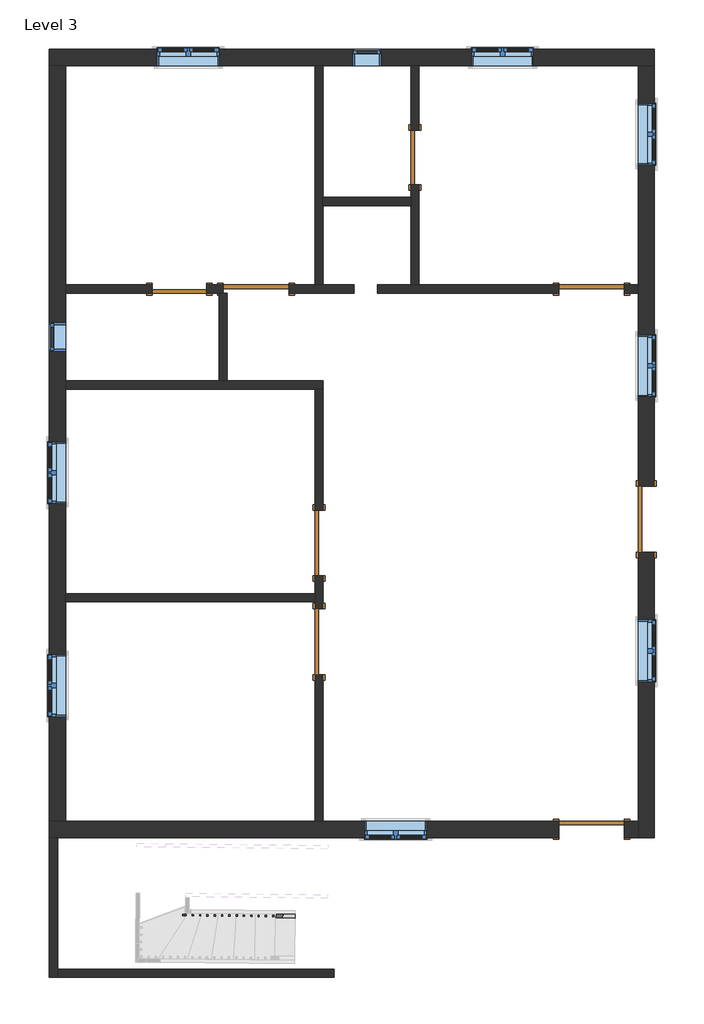
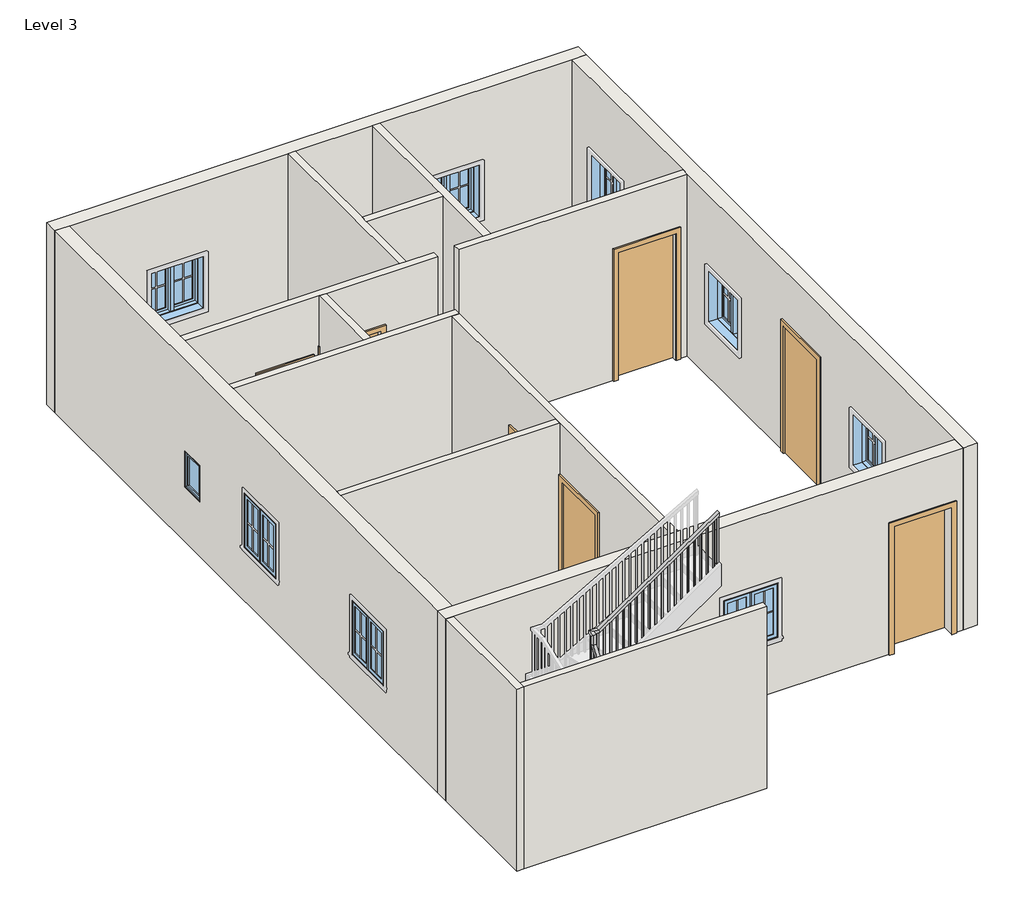
# One storey, part 1 of 2: 15 walls, 10 windows, 8 doors, 1 railing.
"""IFC4 building model written with IfcOpenShell, lengths in millimetres."""

from ifc_helpers import new_model, si_unit, frame, origin, place, context, project, spatial, polyline, outline, extrude, faceted_brep, transform, mapped, element, save
from components import door_f2b275c1, door_e5f9f3c4, door_305aa2a5, door_a90ba1ad, door_0ca8825f, window_aa618e30, window_339605e1

model = new_model("IFC4")

# Units and contexts
model_context = context("Model", 3, world=origin())
ifc_project = project(units=[si_unit("LENGTHUNIT", "METRE", prefix="MILLI")], contexts=[model_context])

# Site, building, storey
site = spatial("IfcSite", under=ifc_project)
building = spatial("IfcBuilding", under=site)
storey = spatial("IfcBuildingStorey", under=building, Name="Level 3", Elevation=3200.4)

# Doors
placement = place(None, origin())
door_shape = door_f2b275c1(model_context)
element("IfcDoor", 1, ObjectType="Single-Flush : 30\" x 80\"", at=placement, inside=storey, context=model_context, shape_type="MappedRepresentation", body=[
    mapped(door_shape, transform((-295.4747832, 5557.2532079, 3200.4), x_axis=(0.0, -1.0, 0.0), y_axis=(1.0, 0.0, 0.0), z_axis=(0.0, 0.0, 1.0))),
])
element("IfcDoor", 2, ObjectType="Single-Flush : 30\" x 80\"", at=placement, inside=storey, context=model_context, shape_type="MappedRepresentation", body=[
    mapped(door_shape, transform((-3572.0747832, 3728.4532079, 3200.4), x_axis=(1.0, 0.0, 0.0), y_axis=(0.0, 1.0, 0.0), z_axis=(0.0, 0.0, 1.0))),
])
door_2_shape = door_e5f9f3c4(model_context)
element("IfcDoor", 3, ObjectType="Single-Flush : 36\" x 84\"", at=placement, inside=storey, context=model_context, shape_type="MappedRepresentation", body=[
    mapped(door_2_shape, transform((-2505.2747832, 3728.4532079, 3200.4), x_axis=(1.0, 0.0, 0.0), y_axis=(0.0, 1.0, 0.0), z_axis=(0.0, 0.0, 1.0))),
])
element("IfcDoor", 4, ObjectType="Single-Flush : 36\" x 84\"", at=placement, inside=storey, context=model_context, shape_type="MappedRepresentation", body=[
    mapped(door_2_shape, transform((2161.9752168, 3728.4532079, 3200.4), x_axis=(1.0, 0.0, 0.0), y_axis=(0.0, 1.0, 0.0), z_axis=(0.0, 0.0, 1.0))),
])
element("IfcDoor", 5, ObjectType="Single-Flush : 36\" x 84\"", at=placement, inside=storey, context=model_context, shape_type="MappedRepresentation", body=[
    mapped(door_2_shape, transform((-1628.9747832, -1173.7467921, 3200.4), x_axis=(0.0, 1.0, 0.0), y_axis=(-1.0, 0.0, 0.0), z_axis=(0.0, 0.0, 1.0))),
])
door_3_shape = door_305aa2a5(model_context)
element("IfcDoor", 6, ObjectType="Single-Flush : 36\" x 84\"", at=placement, inside=storey, context=model_context, shape_type="MappedRepresentation", body=[
    mapped(door_3_shape, transform((-1628.9747832, 197.8532079, 3200.4), x_axis=(0.0, -1.0, 0.0), y_axis=(1.0, 0.0, 0.0), z_axis=(0.0, 0.0, 1.0))),
])
door_4_shape = door_a90ba1ad(model_context)
element("IfcDoor", 7, ObjectType="Single-Flush : 36\" x 84\"", at=placement, inside=storey, context=model_context, shape_type="MappedRepresentation", body=[
    mapped(door_4_shape, transform((2923.9752168, 528.0532079, 3200.4), x_axis=(0.0, -1.0, 0.0), y_axis=(1.0, 0.0, 0.0), z_axis=(0.0, 0.0, 1.0))),
])
door_5_shape = door_0ca8825f(model_context)
element("IfcDoor", 8, ObjectType="Single-Flush : 36\" x 84\"", at=placement, inside=storey, context=model_context, shape_type="MappedRepresentation", body=[
    mapped(door_5_shape, transform((2161.9752168, -3783.5967921, 3200.4), x_axis=(1.0, 0.0, 0.0), y_axis=(0.0, 1.0, 0.0), z_axis=(0.0, 0.0, 1.0))),
])

# Railing
element("IfcRailing", 9, ObjectType="Handrail - Rectangular", at=placement, inside=storey, context=model_context, shape_type="SolidModel", body=[
    faceted_brep([(-1962.1803506, -5016.2038017, 4284.1333333), (-1962.1803506, -5016.2038017, 4222.6793596), (-1961.6349602, -4965.4067295, 4222.6793596), (-1961.6349602, -4965.4067295, 4284.1333333), (-3413.6283866, -5000.6201116, 5272.2756169), (-3464.4254588, -5000.0747212, 5245.4041661), (-3463.8800684, -4949.2776489, 5245.4041661), (-3413.0829962, -4949.8230393, 5272.2756169), (-3413.6283866, -5000.6201116, 5489.361538), (-3464.4254588, -5000.0747212, 5438.561538), (-3463.8800684, -4949.2776489, 5438.561538), (-3413.0829962, -4949.8230393, 5489.361538), (-3540.6210672, -4999.2566356, 5489.361538), (-3540.6210672, -4999.2566356, 5438.561538), (-3489.2786045, -4949.0049537, 5438.561538), (-3489.2786045, -4949.0049537, 5489.361538), (-3539.2575912, -4872.2639549, 5489.361538), (-3538.9677931, -4845.272478, 5438.561538), (-3488.1707209, -4845.8178684, 5438.561538), (-3488.4605189, -4872.8093453, 5489.361538), (-3537.8941152, -4745.2712743, 5677.4249579), (-3537.3487248, -4694.4742021, 5661.8786564), (-3486.5516525, -4695.0195925, 5661.8786564), (-3487.0970429, -4745.8166647, 5677.4249579), (-3537.8941152, -4745.2712743, 5845.476961), (-3537.3487248, -4694.4742021, 5794.676961), (-3486.5516525, -4695.0195925, 5794.676961), (-3487.0970429, -4745.8166647, 5845.476961), (-3536.5306392, -4618.2785937, 5845.476961), (-3536.5306392, -4618.2785937, 5794.676961), (-3486.2789573, -4669.6210563, 5794.676961), (-3486.2789573, -4669.6210563, 5845.476961), (-3409.5379585, -4619.6420697, 5845.476961), (-3393.6525863, -4619.8126254, 5794.676961), (-3394.1979767, -4670.6096976, 5794.676961), (-3410.0833489, -4670.439142, 5845.476961), (-1509.4062983, -4640.0431191, 7162.8), (-1509.9516887, -4690.8401913, 7162.8), (-1509.9516887, -4690.8401913, 7100.9869912), (-1509.4062983, -4640.0431191, 7100.9869912)], [[[0, 1, 2, 3]], [[1, 0, 4, 5]], [[2, 1, 5, 6]], [[3, 2, 6, 7]], [[0, 3, 7, 4]], [[5, 4, 8, 9]], [[6, 5, 9, 10]], [[7, 6, 10, 11]], [[4, 7, 11, 8]], [[9, 8, 12, 13]], [[10, 9, 13, 14]], [[11, 10, 14, 15]], [[8, 11, 15, 12]], [[13, 12, 16, 17]], [[14, 13, 17, 18]], [[15, 14, 18, 19]], [[12, 15, 19, 16]], [[17, 16, 20, 21]], [[18, 17, 21, 22]], [[19, 18, 22, 23]], [[16, 19, 23, 20]], [[21, 20, 24, 25]], [[22, 21, 25, 26]], [[23, 22, 26, 27]], [[20, 23, 27, 24]], [[25, 24, 28, 29]], [[26, 25, 29, 30]], [[27, 26, 30, 31]], [[24, 27, 31, 28]], [[29, 28, 32, 33]], [[30, 29, 33, 34]], [[31, 30, 34, 35]], [[28, 31, 35, 32]], [[36, 37, 38, 39]], [[33, 32, 36, 39]], [[34, 33, 39, 38]], [[35, 34, 38, 37]], [[32, 35, 37, 36]]]),
    extrude(outline(polyline([(221.9968897, -19.05), (235.2031102, 0.0), (1200.994449, 0.0), (1200.994449, -19.05), (221.9968897, -19.05)])), frame((-1590.7427644, -4674.0968508, 7280.0611157), z_axis=(0.01073603161956521, 0.9999423671517594, 0.0), x_axis=(0.0, 0.0, -1.0)), (0.0, 0.0, 1.0), 19.05),
    extrude(outline(polyline([(221.9968898, -19.05), (235.2031102, 0.0), (1130.5612733, 0.0), (1130.5612733, -19.05), (221.9968898, -19.05)])), frame((-1692.3369089, -4673.00607, 7209.62794), z_axis=(0.01073603161956521, 0.9999423671517594, 0.0), x_axis=(0.0, 0.0, -1.0)), (0.0, 0.0, 1.0), 19.05),
    extrude(outline(polyline([(221.9968897, -19.05), (235.2031102, 0.0), (1060.1280975, 0.0), (1060.1280975, -19.05), (221.9968897, -19.05)])), frame((-1793.9310534, -4671.9152892, 7139.1947642), z_axis=(0.01073603161956521, 0.9999423671517594, 0.0), x_axis=(0.0, 0.0, -1.0)), (0.0, 0.0, 1.0), 19.05),
    extrude(outline(polyline([(221.9968898, -19.05), (235.2031103, 0.0), (1159.0282552, 0.0), (1159.0282552, -19.05), (221.9968898, -19.05)])), frame((-1895.5251979, -4670.8245084, 7068.7615885), z_axis=(0.01073603161956521, 0.9999423671517594, 0.0), x_axis=(0.0, 0.0, -1.0)), (0.0, 0.0, 1.0), 19.05),
    extrude(outline(polyline([(221.9968898, -19.05), (235.2031102, 0.0), (1088.5950794, 0.0), (1088.5950794, -19.05), (221.9968898, -19.05)])), frame((-1997.1193424, -4669.7337275, 6998.3284127), z_axis=(0.01073603161956521, 0.9999423671517594, 0.0), x_axis=(0.0, 0.0, -1.0)), (0.0, 0.0, 1.0), 19.05),
    extrude(outline(polyline([(221.9968898, -19.05), (235.2031103, 0.0), (1187.495237, 0.0), (1187.495237, -19.05), (221.9968898, -19.05)])), frame((-2098.7134869, -4668.6429467, 6927.895237), z_axis=(0.01073603161956521, 0.9999423671517594, 0.0), x_axis=(0.0, 0.0, -1.0)), (0.0, 0.0, 1.0), 19.05),
    extrude(outline(polyline([(221.9968898, -19.05), (235.2031102, 0.0), (1117.0620612, 0.0), (1117.0620612, -19.05), (221.9968898, -19.05)])), frame((-2200.3076314, -4667.5521659, 6857.4620612), z_axis=(0.01073603161956521, 0.9999423671517594, 0.0), x_axis=(0.0, 0.0, -1.0)), (0.0, 0.0, 1.0), 19.05),
    extrude(outline(polyline([(221.9968897, -19.0499999), (235.2031102, 0.0), (1046.6288854, 0.0), (1046.6288854, -19.0499999), (221.9968897, -19.0499999)])), frame((-2301.9017759, -4666.4613851, 6787.0288854), z_axis=(0.01073603161956521, 0.9999423671517594, 0.0), x_axis=(0.0, 0.0, -1.0)), (0.0, 0.0, 1.0), 19.05),
    extrude(outline(polyline([(221.9968898, -19.0499999), (235.2031102, 0.0), (1145.529043, 0.0), (1145.529043, -19.0499999), (221.9968898, -19.0499999)])), frame((-2403.4959204, -4665.3706043, 6716.5957097), z_axis=(0.01073603161956521, 0.9999423671517594, 0.0), x_axis=(0.0, 0.0, -1.0)), (0.0, 0.0, 1.0), 19.05),
    extrude(outline(polyline([(221.9968897, -19.05), (235.2031102, 0.0), (1075.0958672, 0.0), (1075.0958672, -19.05), (221.9968897, -19.05)])), frame((-2505.090065, -4664.2798235, 6646.1625339), z_axis=(0.01073603161956521, 0.9999423671517594, 0.0), x_axis=(0.0, 0.0, -1.0)), (0.0, 0.0, 1.0), 19.05),
    extrude(outline(polyline([(221.9968898, -19.05), (235.2031103, 0.0), (1004.6626915, 0.0), (1004.6626915, -19.05), (221.9968898, -19.05)])), frame((-2606.6842095, -4663.1890427, 6575.7293582), z_axis=(0.01073603161956521, 0.9999423671517594, 0.0), x_axis=(0.0, 0.0, -1.0)), (0.0, 0.0, 1.0), 19.05),
    extrude(outline(polyline([(221.9968898, -19.05), (235.2031102, 0.0), (1103.5628491, 0.0), (1103.5628491, -19.05), (221.9968898, -19.05)])), frame((-2708.278354, -4662.0982619, 6505.2961824), z_axis=(0.01073603161956521, 0.9999423671517594, 0.0), x_axis=(0.0, 0.0, -1.0)), (0.0, 0.0, 1.0), 19.05),
    extrude(outline(polyline([(221.9968898, -19.05), (235.2031103, 0.0), (1033.1296734, 0.0), (1033.1296734, -19.05), (221.9968898, -19.05)])), frame((-2809.8724985, -4661.007481, 6434.8630067), z_axis=(0.01073603161956521, 0.9999423671517594, 0.0), x_axis=(0.0, 0.0, -1.0)), (0.0, 0.0, 1.0), 19.05),
    extrude(outline(polyline([(221.9968898, -19.05), (235.2031102, 0.0), (1132.0298309, 0.0), (1132.0298309, -19.05), (221.9968898, -19.05)])), frame((-2911.466643, -4659.9167002, 6364.4298309), z_axis=(0.01073603161956521, 0.9999423671517594, 0.0), x_axis=(0.0, 0.0, -1.0)), (0.0, 0.0, 1.0), 19.05),
    extrude(outline(polyline([(221.9968897, -19.05), (235.2031102, 0.0), (1061.5966551, 0.0), (1061.5966551, -19.05), (221.9968897, -19.05)])), frame((-3013.0607875, -4658.8259194, 6293.9966551), z_axis=(0.01073603161956521, 0.9999423671517594, 0.0), x_axis=(0.0, 0.0, -1.0)), (0.0, 0.0, 1.0), 19.05),
    extrude(outline(polyline([(221.9968898, -19.05), (235.2031102, 0.0), (991.1634794, 0.0), (991.1634794, -19.05), (221.9968898, -19.05)])), frame((-3114.654932, -4657.7351386, 6223.5634794), z_axis=(0.01073603161956521, 0.9999423671517594, 0.0), x_axis=(0.0, 0.0, -1.0)), (0.0, 0.0, 1.0), 19.05),
    extrude(outline(polyline([(221.9968897, -19.05), (235.2031102, 0.0), (1090.0636369, 0.0), (1090.0636369, -19.05), (221.9968897, -19.05)])), frame((-3216.2490765, -4656.6443578, 6153.1303036), z_axis=(0.01073603161956521, 0.9999423671517594, 0.0), x_axis=(0.0, 0.0, -1.0)), (0.0, 0.0, 1.0), 19.05),
    extrude(outline(polyline([(221.9968898, -19.05), (235.2031103, 0.0), (1019.6304612, 0.0), (1019.6304612, -19.05), (221.9968898, -19.05)])), frame((-3317.843221, -4655.553577, 6082.6971279), z_axis=(0.01073603161956521, 0.9999423671517594, 0.0), x_axis=(0.0, 0.0, -1.0)), (0.0, 0.0, 1.0), 19.05),
    extrude(outline(polyline([(221.9968898, -19.05), (235.2031102, 0.0), (1118.5306188, 0.0), (1118.5306188, -19.05), (221.9968898, -19.05)])), frame((-3419.4373655, -4654.4627962, 6012.2639521), z_axis=(0.01073603161956521, 0.9999423671517594, 0.0), x_axis=(0.0, 0.0, -1.0)), (0.0, 0.0, 1.0), 19.05),
    extrude(outline(polyline([(-3502.2553031, -4678.9750729), (-3521.3042052, -4678.7705515), (-3521.0996838, -4659.7216494), (-3502.0507817, -4659.9261708), (-3502.2553031, -4678.9750729)])), frame((0.0, 0.0, 4724.4), z_axis=(0.0, 0.0, 1.0), x_axis=(1.0, 0.0, 0.0)), (0.0, 0.0, 1.0), 1070.276961),
    extrude(outline(polyline([(214.4952435, -19.05), (242.7047565, 0.0), (1222.5739377, 0.0), (1222.5739377, -19.05), (214.4952435, -19.05)])), frame((-3503.3460839, -4780.5692174, 5777.6406044), z_axis=(-0.9999423671517594, 0.010736031619565895, 0.0), x_axis=(0.0, 0.0, -1.0)), (0.0, 0.0, 1.0), 19.05),
    extrude(outline(polyline([(214.4952435, -19.05), (242.7047565, 0.0), (1072.1232018, 0.0), (1072.1232018, -19.05), (214.4952435, -19.05)])), frame((-3504.4368647, -4882.1633619, 5627.1898685), z_axis=(-0.9999423671517594, 0.010736031619565895, 0.0), x_axis=(0.0, 0.0, -1.0)), (0.0, 0.0, 1.0), 19.05),
    extrude(outline(polyline([(-3476.1931112, -4965.0213631), (-3476.3976326, -4984.0702652), (-3495.4465347, -4983.8657438), (-3495.2420133, -4964.8168417), (-3476.1931112, -4965.0213631)])), frame((0.0, 0.0, 4385.7333333), z_axis=(0.0, 0.0, 1.0), x_axis=(1.0, 0.0, 0.0)), (0.0, 0.0, 1.0), 1052.8282047),
    extrude(outline(polyline([(235.0842231, -19.05), (222.115777, 0.0), (1203.1900014, 0.0), (1203.1900014, -19.05), (235.0842231, -19.05)])), frame((-3393.8523902, -4984.9565246, 5419.5900014), z_axis=(0.01073603161956537, 0.9999423671517593, 0.0), x_axis=(0.0, 0.0, -1.0)), (0.0, 0.0, 1.0), 19.05),
    extrude(outline(polyline([(235.084223, -19.05), (222.1157769, 0.0), (1134.0249555, 0.0), (1134.0249555, -19.05), (235.084223, -19.05)])), frame((-3292.2582457, -4986.0473054, 5350.4249555), z_axis=(0.01073603161956537, 0.9999423671517593, 0.0), x_axis=(0.0, 0.0, -1.0)), (0.0, 0.0, 1.0), 19.05),
    extrude(outline(polyline([(235.0842231, -19.05), (222.115777, 0.0), (1234.193243, 0.0), (1234.193243, -19.05), (235.0842231, -19.05)])), frame((-3190.6641012, -4987.1380862, 5281.2599097), z_axis=(0.01073603161956537, 0.9999423671517593, 0.0), x_axis=(0.0, 0.0, -1.0)), (0.0, 0.0, 1.0), 19.05),
    extrude(outline(polyline([(235.084223, -19.05), (222.1157769, 0.0), (1165.0281971, 0.0), (1165.0281971, -19.05), (235.084223, -19.05)])), frame((-3089.0699567, -4988.228867, 5212.0948638), z_axis=(0.01073603161956537, 0.9999423671517593, 0.0), x_axis=(0.0, 0.0, -1.0)), (0.0, 0.0, 1.0), 19.05),
    extrude(outline(polyline([(235.084223, -19.05), (222.1157769, 0.0), (1265.1964847, 0.0), (1265.1964847, -19.05), (235.084223, -19.05)])), frame((-2987.4758122, -4989.3196478, 5142.929818), z_axis=(0.01073603161956537, 0.9999423671517593, 0.0), x_axis=(0.0, 0.0, -1.0)), (0.0, 0.0, 1.0), 19.05),
    extrude(outline(polyline([(235.0842231, -19.05), (222.115777, 0.0), (1196.0314389, 0.0), (1196.0314389, -19.05), (235.0842231, -19.05)])), frame((-2885.8816677, -4990.4104286, 5073.7647722), z_axis=(0.01073603161956537, 0.9999423671517593, 0.0), x_axis=(0.0, 0.0, -1.0)), (0.0, 0.0, 1.0), 19.05),
    extrude(outline(polyline([(235.084223, -19.05), (222.1157769, 0.0), (1296.1997263, 0.0), (1296.1997263, -19.05), (235.084223, -19.05)])), frame((-2784.2875232, -4991.5012094, 5004.5997263), z_axis=(0.01073603161956537, 0.9999423671517593, 0.0), x_axis=(0.0, 0.0, -1.0)), (0.0, 0.0, 1.0), 19.05),
    extrude(outline(polyline([(235.0842231, -19.05), (222.115777, 0.0), (1227.0346805, 0.0), (1227.0346805, -19.05), (235.0842231, -19.05)])), frame((-2682.6933787, -4992.5919903, 4935.4346805), z_axis=(0.01073603161956537, 0.9999423671517593, 0.0), x_axis=(0.0, 0.0, -1.0)), (0.0, 0.0, 1.0), 19.05),
    extrude(outline(polyline([(235.084223, -19.05), (222.1157769, 0.0), (1157.8696346, 0.0), (1157.8696346, -19.05), (235.084223, -19.05)])), frame((-2581.0992342, -4993.6827711, 4866.2696346), z_axis=(0.01073603161956537, 0.9999423671517593, 0.0), x_axis=(0.0, 0.0, -1.0)), (0.0, 0.0, 1.0), 19.05),
    extrude(outline(polyline([(235.0842231, -19.05), (222.115777, 0.0), (1258.0379221, 0.0), (1258.0379221, -19.05), (235.0842231, -19.05)])), frame((-2479.5050897, -4994.7735519, 4797.1045888), z_axis=(0.01073603161956537, 0.9999423671517593, 0.0), x_axis=(0.0, 0.0, -1.0)), (0.0, 0.0, 1.0), 19.05),
    extrude(outline(polyline([(235.084223, -19.05), (222.1157769, 0.0), (1188.8728762, 0.0), (1188.8728762, -19.05), (235.084223, -19.05)])), frame((-2377.9109452, -4995.8643327, 4727.9395429), z_axis=(0.01073603161956537, 0.9999423671517593, 0.0), x_axis=(0.0, 0.0, -1.0)), (0.0, 0.0, 1.0), 19.05),
    extrude(outline(polyline([(235.084223, -19.05), (222.115777, 0.0), (1119.7078304, 0.0), (1119.7078304, -19.05), (235.084223, -19.05)])), frame((-2276.3168007, -4996.9551135, 4658.7744971), z_axis=(0.01073603161956537, 0.9999423671517593, 0.0), x_axis=(0.0, 0.0, -1.0)), (0.0, 0.0, 1.0), 19.05),
    extrude(outline(polyline([(235.0842231, -19.05), (222.115777, 0.0), (1219.876118, 0.0), (1219.876118, -19.05), (235.0842231, -19.05)])), frame((-2174.7226562, -4998.0458943, 4589.6094513), z_axis=(0.01073603161956537, 0.9999423671517593, 0.0), x_axis=(0.0, 0.0, -1.0)), (0.0, 0.0, 1.0), 19.05),
    extrude(outline(polyline([(235.084223, -19.05), (222.1157769, 0.0), (1150.7110721, 0.0), (1150.7110721, -19.05), (235.084223, -19.05)])), frame((-2073.1285117, -4999.1366751, 4520.4444054), z_axis=(0.01073603161956537, 0.9999423671517593, 0.0), x_axis=(0.0, 0.0, -1.0)), (0.0, 0.0, 1.0), 19.05),
    extrude(outline(polyline([(-3501.9826079, -4653.5765368), (-3521.03151, -4653.3720154), (-3520.8269886, -4634.3231133), (-3501.7780865, -4634.5276347), (-3501.9826079, -4653.5765368)])), frame((0.0, 0.0, 4724.4), z_axis=(0.0, 0.0, 1.0), x_axis=(1.0, 0.0, 0.0)), (0.0, 0.0, 1.0), 1070.276961),
    extrude(outline(polyline([(-3505.3231241, -4964.7086043), (-3505.5276455, -4983.7575064), (-3524.5765476, -4983.552985), (-3524.3720262, -4964.5040829), (-3505.3231241, -4964.7086043)])), frame((0.0, 0.0, 4385.7333333), z_axis=(0.0, 0.0, 1.0), x_axis=(1.0, 0.0, 0.0)), (0.0, 0.0, 1.0), 1052.8282047),
    extrude(outline(polyline([(221.9968897, -19.05), (235.2031102, 0.0), (1243.9172142, 0.0), (1243.9172142, -19.05), (221.9968897, -19.05)])), frame((-1528.8301563, -4674.7615848, 7322.9838809), z_axis=(0.01073603161956521, 0.9999423671517594, 0.0), x_axis=(0.0, 0.0, -1.0)), (0.0, 0.0, 1.0), 19.05),
    extrude(outline(polyline([(235.084223, -19.05), (222.1157769, 0.0), (1088.0302493, 0.0), (1088.0302493, -19.05), (235.084223, -19.05)])), frame((-1981.0588182, -5000.1251952, 4457.7635826), z_axis=(0.01073603161956537, 0.9999423671517593, 0.0), x_axis=(0.0, 0.0, -1.0)), (0.0, 0.0, 1.0), 19.05),
])

# Walls
element("IfcWall", 10, ObjectType="WALL4.5\"", at=placement, inside=storey, context=model_context, shape_type="Brep", body=[
    faceted_brep([(-2048.0747832, 3671.3032079, 5334.0), (-2048.0747832, 3671.3032079, 3200.4), (-1141.0287494, 3671.3032079, 3200.4), (-1141.0287494, 3671.3032079, 6248.4), (-2905.3247832, 3671.3032079, 6248.4), (-3019.6247832, 3671.3032079, 6248.4), (-5153.2247832, 3671.3032079, 6248.4), (-5153.2247832, 3671.3032079, 3200.4), (-3953.0747832, 3671.3032079, 3200.4), (-3953.0747832, 3671.3032079, 5232.4), (-3191.0747832, 3671.3032079, 5232.4), (-3191.0747832, 3671.3032079, 3200.4), (-3019.6247832, 3671.3032079, 3200.4), (-2962.4747832, 3671.3032079, 3200.4), (-2962.4747832, 3671.3032079, 5334.0), (-1141.0287494, 3785.6032079, 3200.4), (-1571.8247832, 3785.6032079, 3200.4), (-1686.1247832, 3785.6032079, 3200.4), (-2048.0747832, 3785.6032079, 3200.4), (-2048.0747832, 3785.6032079, 5334.0), (-2962.4747832, 3785.6032079, 5334.0), (-2962.4747832, 3785.6032079, 3200.4), (-3191.0747832, 3785.6032079, 3200.4), (-3191.0747832, 3785.6032079, 5232.4), (-3953.0747832, 3785.6032079, 5232.4), (-3953.0747832, 3785.6032079, 3200.4), (-5153.2247832, 3785.6032079, 3200.4), (-5153.2247832, 3785.6032079, 6248.4), (-1686.1247832, 3785.6032079, 6248.4), (-1571.8247832, 3785.6032079, 6248.4), (-1141.0287494, 3785.6032079, 6248.4)], [[[0, 1, 2, 3, 4, 5, 6, 7, 8, 9, 10, 11, 12, 13, 14]], [[15, 16, 17, 18, 19, 20, 21, 22, 23, 24, 25, 26, 27, 28, 29, 30]], [[8, 7, 26, 25]], [[2, 1, 18, 17, 16, 15]], [[13, 12, 11, 22, 21]], [[3, 2, 15, 30]], [[7, 6, 27, 26]], [[23, 22, 11, 10]], [[24, 23, 10, 9]], [[25, 24, 9, 8]], [[19, 18, 1, 0]], [[20, 19, 0, 14]], [[21, 20, 14, 13]], [[6, 5, 4, 3, 30, 29, 28, 27]]]),
])
element("IfcWall", 11, ObjectType="WALL4.5\"", at=placement, inside=storey, context=model_context, shape_type="Brep", body=[
    faceted_brep([(2619.1752168, 3671.3032079, 5334.0), (2619.1752168, 3671.3032079, 3200.4), (2809.6752168, 3671.3032079, 3200.4), (2809.6752168, 3671.3032079, 6248.4), (-812.7163761, 3671.3032079, 6248.4), (-812.7163761, 3671.3032079, 3200.4), (1704.7752168, 3671.3032079, 3200.4), (1704.7752168, 3671.3032079, 5334.0), (2809.6752168, 3785.6032079, 3200.4), (2619.1752168, 3785.6032079, 3200.4), (2619.1752168, 3785.6032079, 5334.0), (1704.7752168, 3785.6032079, 5334.0), (1704.7752168, 3785.6032079, 3200.4), (-238.3247832, 3785.6032079, 3200.4), (-352.6247832, 3785.6032079, 3200.4), (-812.7163761, 3785.6032079, 3200.4), (-812.7163761, 3785.6032079, 6248.4), (-352.6247832, 3785.6032079, 6248.4), (-238.3247832, 3785.6032079, 6248.4), (2809.6752168, 3785.6032079, 6248.4)], [[[0, 1, 2, 3, 4, 5, 6, 7]], [[8, 9, 10, 11, 12, 13, 14, 15, 16, 17, 18, 19]], [[6, 5, 15, 14, 13, 12]], [[2, 1, 9, 8]], [[5, 4, 16, 15]], [[3, 2, 8, 19]], [[10, 9, 1, 0]], [[11, 10, 0, 7]], [[12, 11, 7, 6]], [[4, 3, 19, 18, 17, 16]]]),
])
element("IfcWall", 12, ObjectType="WALL4.5\"", at=placement, inside=storey, context=model_context, shape_type="Brep", body=[
    faceted_brep([(-1686.1247832, 6833.6032079, 3200.4), (-1686.1247832, 3785.6032079, 3200.4), (-1686.1247832, 3785.6032079, 6248.4), (-1686.1247832, 6833.6032079, 6248.4), (-1571.8247832, 6833.6032079, 3200.4), (-1571.8247832, 6833.6032079, 6248.4), (-1571.8247832, 5004.8032079, 6248.4), (-1571.8247832, 4890.5032079, 6248.4), (-1571.8247832, 3785.6032079, 6248.4), (-1571.8247832, 3785.6032079, 3200.4), (-1571.8247832, 4890.5032079, 3200.4), (-1571.8247832, 5004.8032079, 3200.4)], [[[0, 1, 2, 3]], [[4, 5, 6, 7, 8, 9, 10, 11]], [[1, 0, 4, 11, 10, 9]], [[0, 3, 5, 4]], [[2, 1, 9, 8]], [[3, 2, 8, 7, 6, 5]]]),
])
element("IfcWall", 13, ObjectType="WALL4.5\"", at=placement, inside=storey, context=model_context, shape_type="SweptSolid", body=[
    extrude(outline(polyline([(-352.6247832, 4890.5032079), (-1571.8247832, 4890.5032079), (-1571.8247832, 5004.8032079), (-352.6247832, 5004.8032079), (-352.6247832, 4890.5032079)])), frame((0.0, 0.0, 3200.4), z_axis=(0.0, 0.0, 1.0), x_axis=(1.0, 0.0, 0.0)), (0.0, 0.0, 1.0), 3048.0),
])
element("IfcWall", 14, ObjectType="WALL4.5\"", at=placement, inside=storey, context=model_context, shape_type="Brep", body=[
    faceted_brep([(-352.6247832, 5176.2532079, 5232.4), (-352.6247832, 5176.2532079, 3200.4), (-352.6247832, 5004.8032079, 3200.4), (-352.6247832, 4890.5032079, 3200.4), (-352.6247832, 3785.6032079, 3200.4), (-352.6247832, 3785.6032079, 6248.4), (-352.6247832, 4890.5032079, 6248.4), (-352.6247832, 5004.8032079, 6248.4), (-352.6247832, 6833.6032079, 6248.4), (-352.6247832, 6833.6032079, 3200.4), (-352.6247832, 5938.2532079, 3200.4), (-352.6247832, 5938.2532079, 5232.4), (-238.3247832, 3785.6032079, 3200.4), (-238.3247832, 5176.2532079, 3200.4), (-238.3247832, 5176.2532079, 5232.4), (-238.3247832, 5938.2532079, 5232.4), (-238.3247832, 5938.2532079, 3200.4), (-238.3247832, 6833.6032079, 3200.4), (-238.3247832, 6833.6032079, 6248.4), (-238.3247832, 3785.6032079, 6248.4)], [[[0, 1, 2, 3, 4, 5, 6, 7, 8, 9, 10, 11]], [[12, 13, 14, 15, 16, 17, 18, 19]], [[10, 9, 17, 16]], [[4, 3, 2, 1, 13, 12]], [[9, 8, 18, 17]], [[5, 4, 12, 19]], [[14, 13, 1, 0]], [[15, 14, 0, 11]], [[16, 15, 11, 10]], [[8, 7, 6, 5, 19, 18]]]),
])
element("IfcWall", 15, ObjectType="WALL4.5\"", at=placement, inside=storey, context=model_context, shape_type="Brep", body=[
    faceted_brep([(-3019.6247832, 3671.3032079, 3200.4), (-3019.6247832, 2452.1032079, 3200.4), (-3019.6247832, 2452.1032079, 6248.4), (-3019.6247832, 3671.3032079, 6248.4), (-2905.3247832, 3671.3032079, 3200.4), (-2905.3247832, 3671.3032079, 6248.4), (-2905.3247832, 2452.1032079, 6248.4), (-2905.3247832, 2452.1032079, 3200.4), (-2962.4747832, 3671.3032079, 3200.4)], [[[0, 1, 2, 3]], [[4, 5, 6, 7]], [[1, 0, 8, 4, 7]], [[0, 3, 5, 4, 8]], [[2, 1, 7, 6]], [[3, 2, 6, 5]]]),
])
element("IfcWall", 16, ObjectType="WALL4.5\"", at=placement, inside=storey, context=model_context, shape_type="Brep", body=[
    faceted_brep([(-5153.2247832, 2337.8032079, 3200.4), (-1686.1247832, 2337.8032079, 3200.4), (-1571.8247832, 2337.8032079, 3200.4), (-1571.8247832, 2337.8032079, 6248.4), (-1686.1247832, 2337.8032079, 6248.4), (-5153.2247832, 2337.8032079, 6248.4), (-5153.2247832, 2452.1032079, 3200.4), (-5153.2247832, 2452.1032079, 6248.4), (-3019.6247832, 2452.1032079, 6248.4), (-2905.3247832, 2452.1032079, 6248.4), (-1571.8247832, 2452.1032079, 6248.4), (-1571.8247832, 2452.1032079, 3200.4), (-2905.3247832, 2452.1032079, 3200.4), (-3019.6247832, 2452.1032079, 3200.4)], [[[0, 1, 2, 3, 4, 5]], [[6, 7, 8, 9, 10, 11, 12, 13]], [[2, 1, 0, 6, 13, 12, 11]], [[0, 5, 7, 6]], [[3, 2, 11, 10]], [[5, 4, 3, 10, 9, 8, 7]]]),
])
element("IfcWall", 17, ObjectType="WALL4.5\"", at=placement, inside=storey, context=model_context, shape_type="Brep", body=[
    faceted_brep([(-1686.1247832, -259.3467921, 3200.4), (-1686.1247832, -506.9967921, 3200.4), (-1686.1247832, -621.2967921, 3200.4), (-1686.1247832, -716.5467921, 3200.4), (-1686.1247832, -716.5467921, 5334.0), (-1686.1247832, -1630.9467921, 5334.0), (-1686.1247832, -1630.9467921, 3200.4), (-1686.1247832, -3669.2967921, 3200.4), (-1686.1247832, -3669.2967921, 6248.4), (-1686.1247832, -621.2967921, 6248.4), (-1686.1247832, -506.9967921, 6248.4), (-1686.1247832, 2337.8032079, 6248.4), (-1686.1247832, 2337.8032079, 3200.4), (-1686.1247832, 655.0532079, 3200.4), (-1686.1247832, 655.0532079, 5334.0), (-1686.1247832, -259.3467921, 5334.0), (-1571.8247832, -716.5467921, 5334.0), (-1571.8247832, -716.5467921, 3200.4), (-1571.8247832, -259.3467921, 3200.4), (-1571.8247832, -259.3467921, 5334.0), (-1571.8247832, 655.0532079, 5334.0), (-1571.8247832, 655.0532079, 3200.4), (-1571.8247832, 2337.8032079, 3200.4), (-1571.8247832, 2337.8032079, 6248.4), (-1571.8247832, -3669.2967921, 6248.4), (-1571.8247832, -3669.2967921, 3200.4), (-1571.8247832, -1630.9467921, 3200.4), (-1571.8247832, -1630.9467921, 5334.0)], [[[0, 1, 2, 3, 4, 5, 6, 7, 8, 9, 10, 11, 12, 13, 14, 15]], [[16, 17, 18, 19, 20, 21, 22, 23, 24, 25, 26, 27]], [[13, 12, 22, 21]], [[26, 25, 7, 6]], [[18, 17, 3, 2, 1, 0]], [[12, 11, 23, 22]], [[8, 7, 25, 24]], [[19, 18, 0, 15]], [[20, 19, 15, 14]], [[21, 20, 14, 13]], [[4, 3, 17, 16]], [[5, 4, 16, 27]], [[6, 5, 27, 26]], [[11, 10, 9, 8, 24, 23]]]),
])
element("IfcWall", 18, ObjectType="WALL4.5\"", at=placement, inside=storey, context=model_context, shape_type="SweptSolid", body=[
    extrude(outline(polyline([(-1686.1247832, -621.2967921), (-5153.2247832, -621.2967921), (-5153.2247832, -506.9967921), (-1686.1247832, -506.9967921), (-1686.1247832, -621.2967921)])), frame((0.0, 0.0, 3200.4), z_axis=(0.0, 0.0, 1.0), x_axis=(1.0, 0.0, 0.0)), (0.0, 0.0, 1.0), 3048.0),
])
element("IfcWall", 19, ObjectType="WALL4.5\"", at=placement, inside=storey, context=model_context, shape_type="Brep", body=[
    faceted_brep([(-5381.8247832, -3897.8967921, 3200.4), (-5381.8247832, -5840.9967921, 3200.4), (-5381.8247832, -5840.9967921, 6248.4), (-5381.8247832, -3897.8967921, 6248.4), (-5267.5247832, -3897.8967921, 3200.4), (-5267.5247832, -3897.8967921, 6248.4), (-5267.5247832, -5726.6967921, 6248.4), (-5267.5247832, -5840.9967921, 6248.4), (-5267.5247832, -5840.9967921, 3200.4), (-5267.5247832, -5726.6967921, 3200.4)], [[[0, 1, 2, 3]], [[4, 5, 6, 7, 8, 9]], [[1, 0, 4, 9, 8]], [[0, 3, 5, 4]], [[2, 1, 8, 7]], [[3, 2, 7, 6, 5]]]),
])
element("IfcWall", 20, ObjectType="WALL4.5\"", at=placement, inside=storey, context=model_context, shape_type="SweptSolid", body=[
    extrude(outline(polyline([(-1419.4247832, -5840.9967921), (-5267.5247832, -5840.9967921), (-5267.5247832, -5726.6967921), (-1419.4247832, -5726.6967921), (-1419.4247832, -5840.9967921)])), frame((0.0, 0.0, 3200.4), z_axis=(0.0, 0.0, 1.0), x_axis=(1.0, 0.0, 0.0)), (0.0, 0.0, 1.0), 3048.0),
])
element("IfcWall", 21, ObjectType="WALL9\"", at=placement, inside=storey, context=model_context, shape_type="Brep", body=[
    faceted_brep([(-5381.8247832, 6833.6032079, 3200.4), (-5153.2247832, 6833.6032079, 3200.4), (-1686.1247832, 6833.6032079, 3200.4), (-1571.8247832, 6833.6032079, 3200.4), (-352.6247832, 6833.6032079, 3200.4), (-238.3247832, 6833.6032079, 3200.4), (2809.6752168, 6833.6032079, 3200.4), (3038.2752168, 6833.6032079, 3200.4), (3038.2752168, 6833.6032079, 6248.4), (2809.6752168, 6833.6032079, 6248.4), (-238.3247832, 6833.6032079, 6248.4), (-352.6247832, 6833.6032079, 6248.4), (-1571.8247832, 6833.6032079, 6248.4), (-1686.1247832, 6833.6032079, 6248.4), (-5153.2247832, 6833.6032079, 6248.4), (-5381.8247832, 6833.6032079, 6248.4), (-759.0247832, 6833.6032079, 4724.4), (-759.0247832, 6833.6032079, 4114.8), (-1165.4247832, 6833.6032079, 4114.8), (-1165.4247832, 6833.6032079, 4724.4), (-3016.4497832, 6833.6032079, 5029.2), (-3016.4497832, 6833.6032079, 4114.8), (-3880.0497832, 6833.6032079, 4114.8), (-3880.0497832, 6833.6032079, 5029.2), (1355.5252168, 6833.6032079, 5029.2), (1355.5252168, 6833.6032079, 4114.8), (491.9252168, 6833.6032079, 4114.8), (491.9252168, 6833.6032079, 5029.2), (-5381.8247832, 7062.2032079, 3200.4), (-5381.8247832, 7062.2032079, 6248.4), (3038.2752168, 7062.2032079, 6248.4), (3038.2752168, 7062.2032079, 3200.4), (-759.0247832, 7062.2032079, 4724.4), (-1165.4247832, 7062.2032079, 4724.4), (-1165.4247832, 7062.2032079, 4114.8), (-759.0247832, 7062.2032079, 4114.8), (-3016.4497832, 7062.2032079, 5029.2), (-3880.0497832, 7062.2032079, 5029.2), (-3880.0497832, 7062.2032079, 4114.8), (-3016.4497832, 7062.2032079, 4114.8), (1355.5252168, 7062.2032079, 5029.2), (491.9252168, 7062.2032079, 5029.2), (491.9252168, 7062.2032079, 4114.8), (1355.5252168, 7062.2032079, 4114.8)], [[[0, 1, 2, 3, 4, 5, 6, 7, 8, 9, 10, 11, 12, 13, 14, 15], [16, 17, 18, 19], [20, 21, 22, 23], [24, 25, 26, 27]], [[28, 29, 30, 31], [32, 33, 34, 35], [36, 37, 38, 39], [40, 41, 42, 43]], [[7, 6, 5, 4, 3, 2, 1, 0, 28, 31]], [[8, 7, 31, 30]], [[0, 15, 29, 28]], [[17, 16, 32, 35]], [[18, 17, 35, 34]], [[19, 18, 34, 33]], [[16, 19, 33, 32]], [[21, 20, 36, 39]], [[22, 21, 39, 38]], [[23, 22, 38, 37]], [[20, 23, 37, 36]], [[25, 24, 40, 43]], [[26, 25, 43, 42]], [[27, 26, 42, 41]], [[24, 27, 41, 40]], [[15, 14, 13, 12, 11, 10, 9, 8, 30, 29]]]),
])
element("IfcWall", 22, ObjectType="WALL9\"", at=placement, inside=storey, context=model_context, shape_type="Brep", body=[
    faceted_brep([(2809.6752168, 70.8532079, 5334.0), (2809.6752168, 70.8532079, 3200.4), (2809.6752168, -3669.2967921, 3200.4), (2809.6752168, -3897.8967921, 3200.4), (2809.6752168, -3897.8967921, 6248.4), (2809.6752168, -3669.2967921, 6248.4), (2809.6752168, 3671.3032079, 6248.4), (2809.6752168, 3785.6032079, 6248.4), (2809.6752168, 6833.6032079, 6248.4), (2809.6752168, 6833.6032079, 3200.4), (2809.6752168, 3785.6032079, 3200.4), (2809.6752168, 3671.3032079, 3200.4), (2809.6752168, 985.2532079, 3200.4), (2809.6752168, 985.2532079, 5334.0), (2809.6752168, 5449.3032079, 5029.2), (2809.6752168, 5449.3032079, 4114.8), (2809.6752168, 6312.9032079, 4114.8), (2809.6752168, 6312.9032079, 5029.2), (2809.6752168, 2229.8532079, 5029.2), (2809.6752168, 2229.8532079, 4114.8), (2809.6752168, 3093.4532079, 4114.8), (2809.6752168, 3093.4532079, 5029.2), (2809.6752168, -1732.5467921, 5029.2), (2809.6752168, -1732.5467921, 4114.8), (2809.6752168, -868.9467921, 4114.8), (2809.6752168, -868.9467921, 5029.2), (3038.2752168, -3897.8967921, 3200.4), (3038.2752168, 70.8532079, 3200.4), (3038.2752168, 70.8532079, 5334.0), (3038.2752168, 985.2532079, 5334.0), (3038.2752168, 985.2532079, 3200.4), (3038.2752168, 6833.6032079, 3200.4), (3038.2752168, 6833.6032079, 6248.4), (3038.2752168, -3897.8967921, 6248.4), (3038.2752168, 5449.3032079, 5029.2), (3038.2752168, 6312.9032079, 5029.2), (3038.2752168, 6312.9032079, 4114.8), (3038.2752168, 5449.3032079, 4114.8), (3038.2752168, 2229.8532079, 5029.2), (3038.2752168, 3093.4532079, 5029.2), (3038.2752168, 3093.4532079, 4114.8), (3038.2752168, 2229.8532079, 4114.8), (3038.2752168, -1732.5467921, 5029.2), (3038.2752168, -868.9467921, 5029.2), (3038.2752168, -868.9467921, 4114.8), (3038.2752168, -1732.5467921, 4114.8)], [[[0, 1, 2, 3, 4, 5, 6, 7, 8, 9, 10, 11, 12, 13], [14, 15, 16, 17], [18, 19, 20, 21], [22, 23, 24, 25]], [[26, 27, 28, 29, 30, 31, 32, 33], [34, 35, 36, 37], [38, 39, 40, 41], [42, 43, 44, 45]], [[3, 2, 1, 27, 26]], [[12, 11, 10, 9, 31, 30]], [[9, 8, 32, 31]], [[4, 3, 26, 33]], [[28, 27, 1, 0]], [[29, 28, 0, 13]], [[30, 29, 13, 12]], [[15, 14, 34, 37]], [[16, 15, 37, 36]], [[17, 16, 36, 35]], [[14, 17, 35, 34]], [[19, 18, 38, 41]], [[20, 19, 41, 40]], [[21, 20, 40, 39]], [[18, 21, 39, 38]], [[23, 22, 42, 45]], [[24, 23, 45, 44]], [[25, 24, 44, 43]], [[22, 25, 43, 42]], [[8, 7, 6, 5, 4, 33, 32]]]),
])
element("IfcWall", 23, ObjectType="WALL9\"", at=placement, inside=storey, context=model_context, shape_type="Brep", body=[
    faceted_brep([(2809.6752168, -3669.2967921, 3200.4), (2619.1752168, -3669.2967921, 3200.4), (2619.1752168, -3669.2967921, 5334.0), (1704.7752168, -3669.2967921, 5334.0), (1704.7752168, -3669.2967921, 3200.4), (-1571.8247832, -3669.2967921, 3200.4), (-1686.1247832, -3669.2967921, 3200.4), (-5153.2247832, -3669.2967921, 3200.4), (-5381.8247832, -3669.2967921, 3200.4), (-5381.8247832, -3669.2967921, 6248.4), (-5153.2247832, -3669.2967921, 6248.4), (-1686.1247832, -3669.2967921, 6248.4), (-1571.8247832, -3669.2967921, 6248.4), (2809.6752168, -3669.2967921, 6248.4), (-993.9747832, -3669.2967921, 5029.2), (-993.9747832, -3669.2967921, 4114.8), (-130.3747832, -3669.2967921, 4114.8), (-130.3747832, -3669.2967921, 5029.2), (2619.1752168, -3897.8967921, 5334.0), (2619.1752168, -3897.8967921, 3200.4), (2809.6752168, -3897.8967921, 3200.4), (2809.6752168, -3897.8967921, 6248.4), (-5267.5247832, -3897.8967921, 6248.4), (-5381.8247832, -3897.8967921, 6248.4), (-5381.8247832, -3897.8967921, 3200.4), (-5267.5247832, -3897.8967921, 3200.4), (1704.7752168, -3897.8967921, 3200.4), (1704.7752168, -3897.8967921, 5334.0), (-993.9747832, -3897.8967921, 5029.2), (-130.3747832, -3897.8967921, 5029.2), (-130.3747832, -3897.8967921, 4114.8), (-993.9747832, -3897.8967921, 4114.8)], [[[0, 1, 2, 3, 4, 5, 6, 7, 8, 9, 10, 11, 12, 13], [14, 15, 16, 17]], [[18, 19, 20, 21, 22, 23, 24, 25, 26, 27], [28, 29, 30, 31]], [[20, 19, 1, 0]], [[26, 25, 24, 8, 7, 6, 5, 4]], [[0, 13, 21, 20]], [[9, 8, 24, 23]], [[2, 1, 19, 18]], [[3, 2, 18, 27]], [[4, 3, 27, 26]], [[15, 14, 28, 31]], [[16, 15, 31, 30]], [[17, 16, 30, 29]], [[14, 17, 29, 28]], [[13, 12, 11, 10, 9, 23, 22, 21]]]),
])
element("IfcWall", 24, ObjectType="WALL9\"", at=placement, inside=storey, context=model_context, shape_type="Brep", body=[
    faceted_brep([(-5153.2247832, -3669.2967921, 3200.4), (-5153.2247832, -621.2967921, 3200.4), (-5153.2247832, -506.9967921, 3200.4), (-5153.2247832, 2337.8032079, 3200.4), (-5153.2247832, 2452.1032079, 3200.4), (-5153.2247832, 3671.3032079, 3200.4), (-5153.2247832, 3785.6032079, 3200.4), (-5153.2247832, 6833.6032079, 3200.4), (-5153.2247832, 6833.6032079, 6248.4), (-5153.2247832, 3785.6032079, 6248.4), (-5153.2247832, 3671.3032079, 6248.4), (-5153.2247832, 2452.1032079, 6248.4), (-5153.2247832, 2337.8032079, 6248.4), (-5153.2247832, -506.9967921, 6248.4), (-5153.2247832, -621.2967921, 6248.4), (-5153.2247832, -3669.2967921, 6248.4), (-5153.2247832, 3264.9032079, 4724.4), (-5153.2247832, 3264.9032079, 4114.8), (-5153.2247832, 2858.5032079, 4114.8), (-5153.2247832, 2858.5032079, 4724.4), (-5153.2247832, 1607.5532079, 5029.2), (-5153.2247832, 1607.5532079, 4114.8), (-5153.2247832, 743.9532079, 4114.8), (-5153.2247832, 743.9532079, 5029.2), (-5153.2247832, -1351.5467921, 5029.2), (-5153.2247832, -1351.5467921, 4114.8), (-5153.2247832, -2215.1467921, 4114.8), (-5153.2247832, -2215.1467921, 5029.2), (-5381.8247832, -3669.2967921, 3200.4), (-5381.8247832, -3669.2967921, 6248.4), (-5381.8247832, 6833.6032079, 6248.4), (-5381.8247832, 6833.6032079, 3200.4), (-5381.8247832, 3264.9032079, 4724.4), (-5381.8247832, 2858.5032079, 4724.4), (-5381.8247832, 2858.5032079, 4114.8), (-5381.8247832, 3264.9032079, 4114.8), (-5381.8247832, 1607.5532079, 5029.2), (-5381.8247832, 743.9532079, 5029.2), (-5381.8247832, 743.9532079, 4114.8), (-5381.8247832, 1607.5532079, 4114.8), (-5381.8247832, -1351.5467921, 5029.2), (-5381.8247832, -2215.1467921, 5029.2), (-5381.8247832, -2215.1467921, 4114.8), (-5381.8247832, -1351.5467921, 4114.8)], [[[0, 1, 2, 3, 4, 5, 6, 7, 8, 9, 10, 11, 12, 13, 14, 15], [16, 17, 18, 19], [20, 21, 22, 23], [24, 25, 26, 27]], [[28, 29, 30, 31], [32, 33, 34, 35], [36, 37, 38, 39], [40, 41, 42, 43]], [[7, 6, 5, 4, 3, 2, 1, 0, 28, 31]], [[8, 7, 31, 30]], [[0, 15, 29, 28]], [[17, 16, 32, 35]], [[18, 17, 35, 34]], [[19, 18, 34, 33]], [[16, 19, 33, 32]], [[21, 20, 36, 39]], [[22, 21, 39, 38]], [[23, 22, 38, 37]], [[20, 23, 37, 36]], [[25, 24, 40, 43]], [[26, 25, 43, 42]], [[27, 26, 42, 41]], [[24, 27, 41, 40]], [[15, 14, 13, 12, 11, 10, 9, 8, 30, 29]]]),
])

# Windows
window_shape = window_aa618e30(model_context)
element("IfcWindow", 25, ObjectType="Fixed : 16\" x 24\"", at=placement, inside=storey, context=model_context, shape_type="MappedRepresentation", body=[
    mapped(window_shape, transform((-924.1247832, 6947.9032079, 3200.4), x_axis=(1.0, 0.0, 0.0), y_axis=(0.0, 1.0, 0.0), z_axis=(0.0, 0.0, 1.0))),
])
element("IfcWindow", 26, ObjectType="Fixed : 16\" x 24\"", at=placement, inside=storey, context=model_context, shape_type="MappedRepresentation", body=[
    mapped(window_shape, transform((-5267.5247832, 3099.8032079, 3200.4), x_axis=(0.0, 1.0, 0.0), y_axis=(-1.0, 0.0, 0.0), z_axis=(0.0, 0.0, 1.0))),
])
window_2_shape = window_339605e1(model_context)
element("IfcWindow", 27, ObjectType="Window-Casement-Double : 34\" x 36\"", at=placement, inside=storey, context=model_context, shape_type="MappedRepresentation", body=[
    mapped(window_2_shape, transform((-3448.2497832, 6947.9032079, 3200.4), x_axis=(1.0, 0.0, 0.0), y_axis=(0.0, 1.0, 0.0), z_axis=(0.0, 0.0, 1.0))),
])
element("IfcWindow", 28, ObjectType="Window-Casement-Double : 34\" x 36\"", at=placement, inside=storey, context=model_context, shape_type="MappedRepresentation", body=[
    mapped(window_2_shape, transform((923.7252168, 6947.9032079, 3200.4), x_axis=(1.0, 0.0, 0.0), y_axis=(0.0, 1.0, 0.0), z_axis=(0.0, 0.0, 1.0))),
])
element("IfcWindow", 29, ObjectType="Window-Casement-Double : 34\" x 36\"", at=placement, inside=storey, context=model_context, shape_type="MappedRepresentation", body=[
    mapped(window_2_shape, transform((2923.9752168, 5881.1032079, 3200.4), x_axis=(0.0, -1.0, 0.0), y_axis=(1.0, 0.0, 0.0), z_axis=(0.0, 0.0, 1.0))),
])
element("IfcWindow", 30, ObjectType="Window-Casement-Double : 34\" x 36\"", at=placement, inside=storey, context=model_context, shape_type="MappedRepresentation", body=[
    mapped(window_2_shape, transform((2923.9752168, 2661.6532079, 3200.4), x_axis=(0.0, -1.0, 0.0), y_axis=(1.0, 0.0, 0.0), z_axis=(0.0, 0.0, 1.0))),
])
element("IfcWindow", 31, ObjectType="Window-Casement-Double : 34\" x 36\"", at=placement, inside=storey, context=model_context, shape_type="MappedRepresentation", body=[
    mapped(window_2_shape, transform((2923.9752168, -1300.7467921, 3200.4), x_axis=(0.0, -1.0, 0.0), y_axis=(1.0, 0.0, 0.0), z_axis=(0.0, 0.0, 1.0))),
])
element("IfcWindow", 32, ObjectType="Window-Casement-Double : 34\" x 36\"", at=placement, inside=storey, context=model_context, shape_type="MappedRepresentation", body=[
    mapped(window_2_shape, transform((-5267.5247832, 1175.7532079, 3200.4), x_axis=(0.0, 1.0, 0.0), y_axis=(-1.0, 0.0, 0.0), z_axis=(0.0, 0.0, 1.0))),
])
element("IfcWindow", 33, ObjectType="Window-Casement-Double : 34\" x 36\"", at=placement, inside=storey, context=model_context, shape_type="MappedRepresentation", body=[
    mapped(window_2_shape, transform((-5267.5247832, -1783.3467921, 3200.4), x_axis=(0.0, 1.0, 0.0), y_axis=(-1.0, 0.0, 0.0), z_axis=(0.0, 0.0, 1.0))),
])
element("IfcWindow", 34, ObjectType="Window-Casement-Double : 34\" x 36\"", at=placement, inside=storey, context=model_context, shape_type="MappedRepresentation", body=[
    mapped(window_2_shape, transform((-562.1747832, -3783.5967921, 3200.4), x_axis=(-1.0, 0.0, 0.0), y_axis=(0.0, -1.0, 0.0), z_axis=(0.0, 0.0, 1.0))),
])

save(model, "model.ifc")

# Revit data of these elements
# Type "Single-Flush : 30\" x 80\""
#   Type Mark = "5"
#   Construction Type Id = "MDOOR"
#   Assembly Code = "C1020"
#   Analytic Construction = "Metal"
#   Thickness = 0' - 2"
#   Heat Transfer Coefficient (U) = 0.651978 BTU/(h·ft²·°F)
#   Height = 6' - 8"
#   Trim Projection Ext = 0' - 1"
#   Trim Projection Int = 0' - 1"
#   Trim Width = 0' - 3"
#   Width = 2' - 6"
#   Define Thermal Properties by = 1
#   Define Thermal Properties by = 1
#   Door Material = Door - Panel
#   Frame Material = Door - Frame
#   Visual Light Transmittance = 0
#   Solar Heat Gain Coefficient = 0
#   Function = (empty or 0)
#   Wall Closure = (empty or 0)
# Type "Single-Flush : 36\" x 84\""
#   Type Mark = "1"
#   Construction Type Id = "MDOOR"
#   Assembly Code = "C1020"
#   Analytic Construction = "Metal"
#   Thickness = 0' - 2"
#   Heat Transfer Coefficient (U) = 0.651978 BTU/(h·ft²·°F)
#   Height = 7' - 0"
#   Trim Projection Ext = 0' - 1"
#   Trim Projection Int = 0' - 1"
#   Trim Width = 0' - 3"
#   Width = 3' - 0"
#   Define Thermal Properties by = 1
#   Define Thermal Properties by = 1
#   Door Material = Door - Panel
#   Frame Material = Door - Frame
#   Visual Light Transmittance = 0
#   Solar Heat Gain Coefficient = 0
#   Function = (empty or 0)
#   Wall Closure = (empty or 0)
# Type "Handrail - Rectangular"
#   Assembly Code = "C2010400"
#   built-in parameter 1008612 = 0.0416667 (stored number, unit not read)
#   built-in parameter 1008611 = 0.0416667 (stored number, unit not read)
#   built-in parameter 1008609 = 0.333333 (stored number, unit not read)
#   built-in parameter 1008604 = 0.166667 (stored number, unit not read)
#   built-in parameter 1008603 = 0.166667 (stored number, unit not read)
#   Railing Height = 3' - 0"
#   built-in parameter 1008630 = 2
#   built-in parameter 1008610 = 2
#   built-in parameter 1008618 = Baluster - Square : 3/4"
# Type "WALL4.5\""
#   Assembly Code = "B2010"
#   Layers, outside or top first: 0' - 4 1/2" no material (function 1)
# Type "WALL9\""
#   Assembly Code = "B2010"
#   Layers, outside or top first: 0' - 9" no material (function 1)
# Type "Fixed : 16\" x 24\""
#   Type Mark = "4"
#   Construction Type Id = "GSP4R"
#   Assembly Code = "B2020100"
#   Analytic Construction = "1/8 in Pilkington single glazing"
#   Visual Light Transmittance = 0.9
#   Solar Heat Gain Coefficient = 0.78
#   Heat Transfer Coefficient (U) = 0.6496 BTU/(h·ft²·°F)
#   Height = 2' - 0"
#   Default Sill Height = 3' - 0"
#   Width = 1' - 4"
#   Window Inset = 0' - 0 3/4"
#   Define Thermal Properties by = 1
#   Define Thermal Properties by = 1
#   Glass Pane Material = Glass
#   Sash Material = Sash
#   Wall Closure = (empty or 0)
# Type "Window-Casement-Double : 34\" x 36\""
#   Type Mark = "14"
#   Fire Rating = "0.5h"
#   Assembly Code = "B2020100"
#   Analytic Construction = "Double glazing - domestic"
#   Frame Extension [instance default] = 0' - 0 1/4"
#   Window Inset [instance default] = 0' - 0"
#   Wall Thickness [instance default] = 0' - 6"
#   Interior Wall Closure [instance default] = 0' - 2 1/4"
#   Half Width = 1' - 5"
#   Visual Light Transmittance = 0.81
#   Thermal Resistance (R) = 1.8146 (h·ft²·°F)/BTU
#   Solar Heat Gain Coefficient = 0.76
#   Rough Width = 2' - 10 1/2"
#   Rough Height = 3' - 0 1/2"
#   Height = 3' - 0"
#   Heat Transfer Coefficient (U) = 0.5511 BTU/(h·ft²·°F)
#   Exterior Wall Closure [instance default] = 0' - 1 1/4"
#   Extension Jamb [instance default] = 0' - 2 1/4"
#   Default Sill Height = 3' - 0"
#   Width = 2' - 10"
#   Define Thermal Properties by = 0
#   Muntin Visibility = yes
#   Interior Trim Visibility [instance default] = yes
#   Exterior Trim Visibility [instance default] = yes
#   Extension Jamb Visibility [instance default] = yes
#   Interior Trim Material = Wood - Stained
#   Muntin Pattern = Muntin Pattern_2x2 : Muntin Pattern_2x2
#   Interior Trim = Trim-Window-Interior-Flat : Picture Frame
#   Interior Frame Material = Wood - Stained
#   Glass Panel Material = Glass
#   Exterior Trim Material = Clad - White
#   Exterior Trim = Trim-Window-Exterior-Flat : with Sill
#   Exterior Frame Material = Clad - White
#   Wall Closure = (empty or 0)
# Elements 1, 2 (IfcDoor, "Single-Flush : 30\" x 80\"")
#   Phase Created = New Construction
#   Materials on its faces: "Door - Frame", "Door - Panel"
# Elements 3, 4, 5, 6, 7, 8 (IfcDoor, "Single-Flush : 36\" x 84\"")
#   Phase Created = New Construction
#   Materials on its faces: "Door - Frame", "Door - Panel"
# Element 9 (IfcRailing, "Handrail - Rectangular")
#   Phase Created = New Construction
# Elements 10, 11, 12, 13, 14, 15, 16, 17, 18 (IfcWall, "WALL4.5\"")
#   Top Offset = 0' - 0"
#   Base Offset = 0' - 0"
#   Unconnected Height = 10' - 0"
#   wall height = 10' - 0"
#   Phase Created = New Construction
#   Base Constraint = Level 3
#   Materials on its faces: "Default Wall"
# Elements 19, 20 (IfcWall, "WALL4.5\"")
#   Top Offset = 0' - 0"
#   Base Offset = 0' - 0"
#   Unconnected Height = 10' - 0"
#   wall height = 10' - 0"
#   Phase Created = New Construction
#   Base Constraint = Level 3
#   Materials on its faces: "Default Wall", "Carpet (1)"
# Elements 21, 22, 23, 24 (IfcWall, "WALL9\"")
#   Top Offset = 0' - 0"
#   Base Offset = 0' - 0"
#   Unconnected Height = 10' - 0"
#   wall height = 10' - 0"
#   Phase Created = New Construction
#   Base Constraint = Level 3
#   Materials on its faces: "Default Wall", "Carpet (1)"
# Element 25 (IfcWindow, "Fixed : 16\" x 24\"")
#   Mark = "11"
#   Phase Created = New Construction
#   Materials on its faces: "Sash", "Glass"
# Element 26 (IfcWindow, "Fixed : 16\" x 24\"")
#   Mark = "12"
#   Phase Created = New Construction
#   Materials on its faces: "Sash", "Glass"
# Element 27 (IfcWindow, "Window-Casement-Double : 34\" x 36\"")
#   Mark = "13"
#   Window Inset = 0' - 0"
#   Interior Wall Closure = 0' - 2 1/4"
#   Frame Extension = 0' - 0 1/4"
#   Exterior Wall Closure = 0' - 1 1/4"
#   Interior Trim Visibility = yes
#   Exterior Trim Visibility = yes
#   Phase Created = New Construction
#   Materials on its faces: "Wood - Stained", "Glass", "Clad - White"
# Element 28 (IfcWindow, "Window-Casement-Double : 34\" x 36\"")
#   Mark = "14"
#   Window Inset = 0' - 0"
#   Interior Wall Closure = 0' - 2 1/4"
#   Frame Extension = 0' - 0 1/4"
#   Exterior Wall Closure = 0' - 1 1/4"
#   Interior Trim Visibility = yes
#   Exterior Trim Visibility = yes
#   Phase Created = New Construction
#   Materials on its faces: "Wood - Stained", "Glass", "Clad - White"
# Element 29 (IfcWindow, "Window-Casement-Double : 34\" x 36\"")
#   Mark = "15"
#   Window Inset = 0' - 0"
#   Interior Wall Closure = 0' - 2 1/4"
#   Frame Extension = 0' - 0 1/4"
#   Exterior Wall Closure = 0' - 1 1/4"
#   Interior Trim Visibility = yes
#   Exterior Trim Visibility = yes
#   Phase Created = New Construction
#   Materials on its faces: "Wood - Stained", "Glass", "Clad - White"
# Element 30 (IfcWindow, "Window-Casement-Double : 34\" x 36\"")
#   Mark = "16"
#   Window Inset = 0' - 0"
#   Interior Wall Closure = 0' - 2 1/4"
#   Frame Extension = 0' - 0 1/4"
#   Exterior Wall Closure = 0' - 1 1/4"
#   Interior Trim Visibility = yes
#   Exterior Trim Visibility = yes
#   Phase Created = New Construction
#   Materials on its faces: "Wood - Stained", "Glass", "Clad - White"
# Element 31 (IfcWindow, "Window-Casement-Double : 34\" x 36\"")
#   Mark = "17"
#   Window Inset = 0' - 0"
#   Interior Wall Closure = 0' - 2 1/4"
#   Frame Extension = 0' - 0 1/4"
#   Exterior Wall Closure = 0' - 1 1/4"
#   Interior Trim Visibility = yes
#   Exterior Trim Visibility = yes
#   Phase Created = New Construction
#   Materials on its faces: "Wood - Stained", "Glass", "Clad - White"
# Element 32 (IfcWindow, "Window-Casement-Double : 34\" x 36\"")
#   Mark = "18"
#   Window Inset = 0' - 0"
#   Interior Wall Closure = 0' - 2 1/4"
#   Frame Extension = 0' - 0 1/4"
#   Exterior Wall Closure = 0' - 1 1/4"
#   Interior Trim Visibility = yes
#   Exterior Trim Visibility = yes
#   Phase Created = New Construction
#   Materials on its faces: "Wood - Stained", "Glass", "Clad - White"
# Element 33 (IfcWindow, "Window-Casement-Double : 34\" x 36\"")
#   Mark = "19"
#   Window Inset = 0' - 0"
#   Interior Wall Closure = 0' - 2 1/4"
#   Frame Extension = 0' - 0 1/4"
#   Exterior Wall Closure = 0' - 1 1/4"
#   Interior Trim Visibility = yes
#   Exterior Trim Visibility = yes
#   Phase Created = New Construction
#   Materials on its faces: "Wood - Stained", "Glass", "Clad - White"
# Element 34 (IfcWindow, "Window-Casement-Double : 34\" x 36\"")
#   Mark = "20"
#   Window Inset = 0' - 0"
#   Interior Wall Closure = 0' - 2 1/4"
#   Frame Extension = 0' - 0 1/4"
#   Exterior Wall Closure = 0' - 1 1/4"
#   Interior Trim Visibility = yes
#   Exterior Trim Visibility = yes
#   Phase Created = New Construction
#   Materials on its faces: "Wood - Stained", "Glass", "Clad - White"
# Materials
#   "Door - Panel": class "Wood", colour RGB 210 159 95, transparency 0, Cost = 0
#   "Door - Frame": colour RGB 118 70 51, transparency 0, Cost = 0
#   "Glass": class "Glass", colour RGB 0 128 192, transparency 0.75, Description = "Soda Lime Glass", Cost = 0
#   "Sash": class "Wood", colour RGB 224 178 126, transparency 0, Cost = 0
#   "Wood - Stained": class "Wood", colour RGB 224 178 126, transparency 0, Cost = 0
#   "Clad - White": class "Wood", colour RGB 242 242 238, transparency 0, Cost = 0
#   "Default Wall": colour RGB 128 128 128, transparency 0, Cost = 0
#   "Carpet (1)": class "Carpet", colour RGB 124 80 67, transparency 0, Description = "Interior finish", Cost = 0
